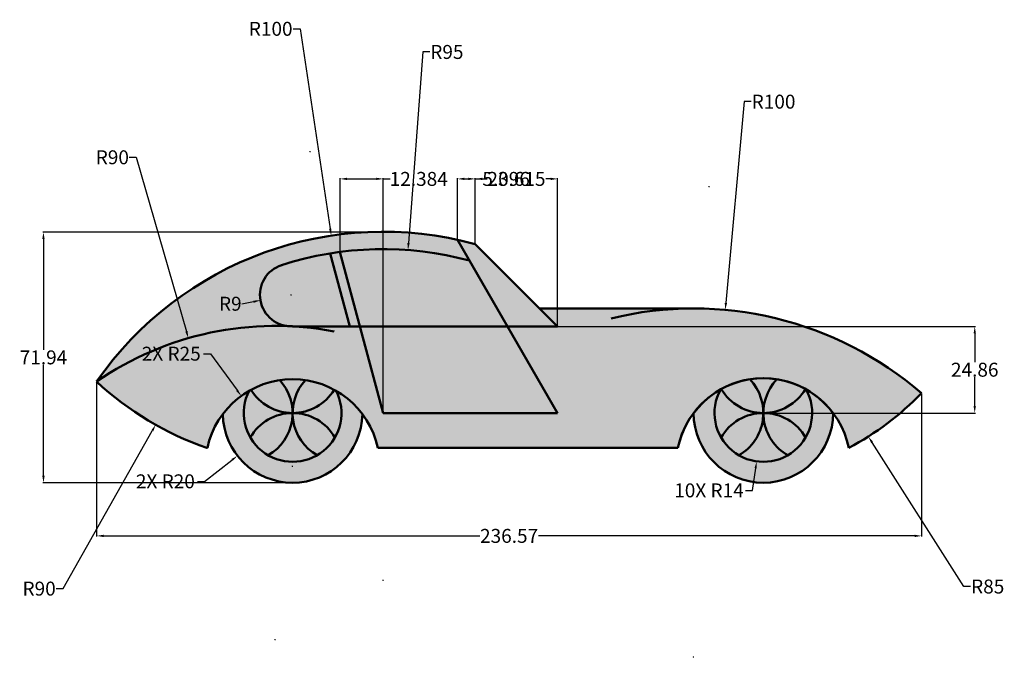
# Model space of a CAD drawing. Units: millimetres. Extents: x -64 to 541, y -54 to 145.
# Tile 2 of 2: x 259 to 541, y -43 to 140. Entities that reach past the tile are written whole.
import ezdxf

# ---------------------------------------------------------------- set-up
doc = ezdxf.new("R2010")
doc.units = ezdxf.units.MM
doc.header["$MEASUREMENT"] = 0
for name, color, linetype, lineweight in [('M-DIMS', 2, 'Continuous', 25), ('M-HATC', 9, 'Continuous', 18), ('M-OUTL', 7, 'Continuous', 50)]:
    doc.layers.add(name, color=color, linetype=linetype, lineweight=lineweight)
doc.styles.get("Standard").update_dxf_attribs({"font": 'arial.ttf'})
doc.dimstyles.get("Standard").update_dxf_attribs({"dimtxt": 4, "dimasz": 2, "dimexe": 0.18, "dimexo": 0.0625, "dimgap": 0.09, "dimtad": 0, "dimtih": 1, "dimtoh": 1, "dimdec": 0, "dimzin": 0, "dimdsep": 46, "dimtxsty": 'Standard', "dimcen": 0.09, "dimadec": 0, "dimazin": 0, "dimtfac": 1, "dimtdec": 0, "dimtofl": 0, "dimtmove": 0, "dimatfit": 3, "dimfxl": 1, "dimtolj": 1, "dimtzin": 0, "dimarcsym": 0})

# ---------------------------------------------------------------- blocks, each defined once
blk = doc.blocks.new('SPORTS-CAR-SIDE-PROFILE')
for p, q in [((132.2, 20), (103.49, 69.73)), ((132.2, 44.86), (108.59, 68.48)), ((72.59, 44.86), (66.98, 65.8)), ((82.17, 20), (69.79, 66.22)), ((171.2, 50), (127.07, 50)), ((56.2, 44.86), (132.2, 44.86)), ((82.17, 20), (132.2, 20)), ((31.62, 10), (31.77, 10)), ((80.64, 10), (166.71, 10))]:
    blk.add_line(p, q)
for centre, radius, start, end in [((82.17, -27.97), 100, 74.6835, 145.2591), ((82.17, -27.97), 95, 74.8819, 107.8414), ((55.83, 53.89), 9, 107.8414, 272.4141), ((171.2, -50), 100, 49.1795, 103.6939), ((51.2, -45), 90, 79.1521, 124.6758), ((61.2, 95), 90, 227.1529, 250.8119), ((56.2, 4.72), 25, 12.189, 167.811), ((42.2, 20), 14, 300, 42.4573), ((70.2, 20), 14, 137.5427, 240), ((191.2, 5), 25, 36.8699, 168.463), ((191.2, 5), 25, 11.537, 168.463), ((177.2, 20), 14, 300, 43.8229), ((205.2, 20), 14, 136.1771, 240), ((56.2, 20), 14, 152.7963, 27.2037), ((56.2, 34), 14, 211.4905, 328.5095), ((191.2, 20), 14, 150.9407, 29.0593), ((191.2, 34), 14, 210.4901, 329.5099), ((175.7, 85), 85, 298.0725, 315.739), ((56.2, 6), 14, 30, 150), ((191.2, 20), 20, 180, 0), ((191.2, 6), 14, 30, 150), ((56.2, 20), 20, 180.7904, 359.2096)]:
    blk.add_arc(centre, radius, start, end)
blk = doc.blocks.new('*D32')
at = {"layer": 'Defpoints', "color": 0, "transparency": 16777216}
for p in [(280.72, 35.85), (517.29, 32.51), (517.29, -8.41)]:
    blk.add_point(p, dxfattribs=at)
at = {"layer": 'M-DIMS', "color": 0, "lineweight": -2, "transparency": 16777216}
for p, q in [((280.72, 35.79), (280.72, -8.59)), ((517.29, 32.45), (517.29, -8.59)), ((282.72, -8.41), (390.58, -8.41)), ((515.29, -8.41), (407.43, -8.41))]:
    blk.add_line(p, q, dxfattribs=at)
at = {"layer": 'M-DIMS', "color": 0, "transparency": 16777216}
for points in [[(282.72, -8.08), (282.72, -8.75), (280.72, -8.41)], [(515.29, -8.08), (515.29, -8.75), (517.29, -8.41)]]:
    blk.add_solid(points, dxfattribs=at)
at = {"layer": 'M-DIMS', "color": 0, "transparency": 16777216, "insert": (399, -8.41), "char_height": 4, "attachment_point": 5}
blk.add_mtext('\\A1;236.57', dxfattribs=at)
blk = doc.blocks.new('*D33')
at = {"layer": 'Defpoints', "color": 0, "transparency": 16777216}
for p in [(265.47, 78.77), (358.48, 78.77), (336.92, 6.84)]:
    blk.add_point(p, dxfattribs=at)
at = {"layer": 'M-DIMS', "color": 0, "lineweight": -2, "transparency": 16777216}
for p, q in [((358.42, 78.77), (265.29, 78.77)), ((265.47, 76.77), (265.47, 44.94)), ((265.47, 8.84), (265.47, 40.67)), ((336.86, 6.84), (265.29, 6.84))]:
    blk.add_line(p, q, dxfattribs=at)
at = {"layer": 'M-DIMS', "color": 0, "transparency": 16777216}
for points in [[(265.13, 76.77), (265.8, 76.77), (265.47, 78.77)], [(265.13, 8.84), (265.8, 8.84), (265.47, 6.84)]]:
    blk.add_solid(points, dxfattribs=at)
at = {"layer": 'M-DIMS', "color": 0, "transparency": 16777216, "insert": (265.47, 42.81), "char_height": 4, "attachment_point": 5}
blk.add_mtext('\\A1;71.94', dxfattribs=at)
blk = doc.blocks.new('*D34')
at = {"layer": 'Defpoints', "color": 0, "transparency": 16777216}
for p in [(362.89, 94.02), (350.51, 73.05), (362.89, 26.84)]:
    blk.add_point(p, dxfattribs=at)
at = {"layer": 'M-DIMS', "color": 0, "lineweight": -2, "transparency": 16777216}
for p, q in [((350.51, 73.12), (350.51, 94.2)), ((352.51, 94.02), (360.89, 94.02)), ((362.89, 26.9), (362.89, 94.2)), ((362.89, 94.02), (364.89, 94.02))]:
    blk.add_line(p, q, dxfattribs=at)
at = {"layer": 'M-DIMS', "color": 0, "transparency": 16777216}
for points in [[(352.51, 94.36), (352.51, 93.69), (350.51, 94.02)], [(360.89, 94.36), (360.89, 93.69), (362.89, 94.02)]]:
    blk.add_solid(points, dxfattribs=at)
at = {"layer": 'M-DIMS', "color": 0, "transparency": 16777216, "insert": (373.09, 94.02), "char_height": 4, "attachment_point": 5}
blk.add_mtext('\\A1;12.384', dxfattribs=at)
blk = doc.blocks.new('*D35')
at = {"layer": 'Defpoints', "color": 0, "transparency": 16777216}
for p in [(389.31, 94.02), (384.21, 76.57), (389.31, 75.31)]:
    blk.add_point(p, dxfattribs=at)
at = {"layer": 'M-DIMS', "color": 0, "lineweight": -2, "transparency": 16777216}
for p, q in [((384.21, 76.63), (384.21, 94.2)), ((386.21, 94.02), (387.31, 94.02)), ((389.31, 75.38), (389.31, 94.2)), ((389.31, 94.02), (391.31, 94.02))]:
    blk.add_line(p, q, dxfattribs=at)
at = {"layer": 'M-DIMS', "color": 0, "transparency": 16777216}
for points in [[(386.21, 94.36), (386.21, 93.69), (384.21, 94.02)], [(387.31, 94.36), (387.31, 93.69), (389.31, 94.02)]]:
    blk.add_solid(points, dxfattribs=at)
at = {"layer": 'M-DIMS', "color": 0, "transparency": 16777216, "insert": (398.14, 94.02), "char_height": 4, "attachment_point": 5}
blk.add_mtext('\\A1;5.096', dxfattribs=at)
blk = doc.blocks.new('*D36')
at = {"layer": 'Defpoints', "color": 0, "transparency": 16777216}
for p in [(412.92, 94.02), (389.31, 75.31), (412.92, 51.7)]:
    blk.add_point(p, dxfattribs=at)
at = {"layer": 'M-DIMS', "color": 0, "lineweight": -2, "transparency": 16777216}
for p, q in [((389.31, 75.38), (389.31, 94.2)), ((391.31, 94.02), (392.67, 94.02)), ((410.92, 94.02), (409.55, 94.02)), ((412.92, 51.76), (412.92, 94.2))]:
    blk.add_line(p, q, dxfattribs=at)
at = {"layer": 'M-DIMS', "color": 0, "transparency": 16777216}
for points in [[(391.31, 94.36), (391.31, 93.69), (389.31, 94.02)], [(410.92, 94.36), (410.92, 93.69), (412.92, 94.02)]]:
    blk.add_solid(points, dxfattribs=at)
at = {"layer": 'M-DIMS', "color": 0, "transparency": 16777216, "insert": (401.11, 94.02), "char_height": 4, "attachment_point": 5}
blk.add_mtext('\\A1;23.615', dxfattribs=at)
blk = doc.blocks.new('*D37')
at = {"layer": 'Defpoints', "color": 0, "transparency": 16777216}
for p in [(412.92, 51.7), (532.54, 51.7), (471.92, 26.84)]:
    blk.add_point(p, dxfattribs=at)
at = {"layer": 'M-DIMS', "color": 0, "lineweight": -2, "transparency": 16777216}
for p, q in [((412.98, 51.7), (532.72, 51.7)), ((532.54, 49.7), (532.54, 41.4)), ((532.54, 28.84), (532.54, 37.14)), ((471.98, 26.84), (532.72, 26.84))]:
    blk.add_line(p, q, dxfattribs=at)
at = {"layer": 'M-DIMS', "color": 0, "transparency": 16777216}
for points in [[(532.21, 49.7), (532.87, 49.7), (532.54, 51.7)], [(532.21, 28.84), (532.87, 28.84), (532.54, 26.84)]]:
    blk.add_solid(points, dxfattribs=at)
at = {"layer": 'M-DIMS', "color": 0, "transparency": 16777216, "insert": (532.54, 39.27), "char_height": 4, "attachment_point": 5}
blk.add_mtext('\\A1;24.86', dxfattribs=at)
blk = doc.blocks.new('*D38')
at = {"layer": 'Defpoints', "color": 0, "transparency": 16777216}
for p in [(322.18, 31.75), (336.92, 11.56)]:
    blk.add_point(p, dxfattribs=at)
at = {"layer": 'M-DIMS', "color": 0, "lineweight": -2, "transparency": 16777216}
for p, q in [((311.34, 43.87), (313.34, 43.87)), ((313.34, 43.87), (321, 33.37)), ((336.83, 11.56), (337.01, 11.56)), ((336.92, 11.47), (336.92, 11.65))]:
    blk.add_line(p, q, dxfattribs=at)
at = {"layer": 'M-DIMS', "color": 0, "transparency": 16777216}
blk.add_solid([(321.27, 33.56), (320.73, 33.17), (322.18, 31.75)], dxfattribs=at)
at = {"layer": 'M-DIMS', "color": 0, "transparency": 16777216, "insert": (302.12, 43.87), "char_height": 4, "attachment_point": 5}
blk.add_mtext('\\A1;2X R25', dxfattribs=at)
blk = doc.blocks.new('*D39')
at = {"layer": 'Defpoints', "color": 0, "transparency": 16777216}
for p in [(336.92, 26.84), (321.11, 14.59)]:
    blk.add_point(p, dxfattribs=at)
at = {"layer": 'M-DIMS', "color": 0, "lineweight": -2, "transparency": 16777216}
for p, q in [((336.83, 26.84), (337.01, 26.84)), ((336.92, 26.75), (336.92, 26.93)), ((311.63, 7.24), (319.53, 13.36)), ((309.63, 7.24), (311.63, 7.24))]:
    blk.add_line(p, q, dxfattribs=at)
at = {"layer": 'M-DIMS', "color": 0, "transparency": 16777216}
blk.add_solid([(319.33, 13.62), (319.73, 13.1), (321.11, 14.59)], dxfattribs=at)
at = {"layer": 'M-DIMS', "color": 0, "transparency": 16777216, "insert": (300.43, 7.24), "char_height": 4, "attachment_point": 5}
blk.add_mtext('\\A1;2X R20', dxfattribs=at)
blk = doc.blocks.new('*D40')
at = {"layer": 'Defpoints', "color": 0, "transparency": 16777216}
for p in [(471.92, 26.84), (470, 12.97)]:
    blk.add_point(p, dxfattribs=at)
at = {"layer": 'M-DIMS', "color": 0, "lineweight": -2, "transparency": 16777216}
for p, q in [((471.83, 26.84), (472.01, 26.84)), ((471.92, 26.75), (471.92, 26.93)), ((468.84, 4.65), (469.72, 10.99)), ((466.84, 4.65), (468.84, 4.65))]:
    blk.add_line(p, q, dxfattribs=at)
at = {"layer": 'M-DIMS', "color": 0, "transparency": 16777216}
blk.add_solid([(469.39, 11.04), (470.05, 10.94), (470, 12.97)], dxfattribs=at)
at = {"layer": 'M-DIMS', "color": 0, "transparency": 16777216, "insert": (456.32, 4.65), "char_height": 4, "attachment_point": 5}
blk.add_mtext('\\A1;10X R14', dxfattribs=at)
blk = doc.blocks.new('*D41')
at = {"layer": 'Defpoints', "color": 0, "transparency": 16777216}
for p in [(336.54, 60.73), (327.68, 59.15)]:
    blk.add_point(p, dxfattribs=at)
at = {"layer": 'M-DIMS', "color": 0, "lineweight": -2, "transparency": 16777216}
for p, q in [((336.45, 60.73), (336.63, 60.73)), ((336.54, 60.64), (336.54, 60.82)), ((322.37, 58.2), (325.71, 58.8))]:
    blk.add_line(p, q, dxfattribs=at)
at = {"layer": 'M-DIMS', "color": 0, "transparency": 16777216}
blk.add_solid([(325.65, 59.12), (325.77, 58.47), (327.68, 59.15)], dxfattribs=at)
at = {"layer": 'M-DIMS', "color": 0, "transparency": 16777216, "insert": (319.05, 58.2), "char_height": 4, "attachment_point": 5}
blk.add_mtext('\\A1;R9', dxfattribs=at)
blk = doc.blocks.new('*D42')
at = {"layer": 'Defpoints', "color": 0, "transparency": 16777216}
for p in [(347.99, 77.75), (362.89, -21.13)]:
    blk.add_point(p, dxfattribs=at)
at = {"layer": 'M-DIMS', "color": 0, "lineweight": -2, "transparency": 16777216}
for p, q in [((337.04, 137.08), (339.04, 137.08)), ((339.04, 137.08), (347.69, 79.73)), ((362.8, -21.13), (362.98, -21.13)), ((362.89, -21.22), (362.89, -21.04))]:
    blk.add_line(p, q, dxfattribs=at)
at = {"layer": 'M-DIMS', "color": 0, "transparency": 16777216}
blk.add_solid([(348.02, 79.78), (347.36, 79.68), (347.99, 77.75)], dxfattribs=at)
at = {"layer": 'M-DIMS', "color": 0, "transparency": 16777216, "insert": (330.63, 137.08), "char_height": 4, "attachment_point": 5}
blk.add_mtext('\\A1;R100', dxfattribs=at)
blk = doc.blocks.new('*D43')
at = {"layer": 'Defpoints', "color": 0, "transparency": 16777216}
for p in [(370.01, 73.6), (362.89, -21.13)]:
    blk.add_point(p, dxfattribs=at)
at = {"layer": 'M-DIMS', "color": 0, "lineweight": -2, "transparency": 16777216}
for p, q in [((374.28, 130.44), (370.16, 75.59)), ((376.28, 130.44), (374.28, 130.44)), ((362.8, -21.13), (362.98, -21.13)), ((362.89, -21.22), (362.89, -21.04))]:
    blk.add_line(p, q, dxfattribs=at)
at = {"layer": 'M-DIMS', "color": 0, "transparency": 16777216}
blk.add_solid([(369.82, 75.62), (370.49, 75.57), (370.01, 73.6)], dxfattribs=at)
at = {"layer": 'M-DIMS', "color": 0, "transparency": 16777216, "insert": (381.16, 130.44), "char_height": 4, "attachment_point": 5}
blk.add_mtext('\\A1;R95', dxfattribs=at)
blk = doc.blocks.new('*D44')
at = {"layer": 'Defpoints', "color": 0, "transparency": 16777216}
for p in [(307.02, 48.32), (331.92, -38.16)]:
    blk.add_point(p, dxfattribs=at)
at = {"layer": 'M-DIMS', "color": 0, "lineweight": -2, "transparency": 16777216}
for p, q in [((290.08, 100.22), (292.08, 100.22)), ((292.08, 100.22), (306.47, 50.25)), ((331.83, -38.16), (332.01, -38.16)), ((331.92, -38.25), (331.92, -38.07))]:
    blk.add_line(p, q, dxfattribs=at)
at = {"layer": 'M-DIMS', "color": 0, "transparency": 16777216}
blk.add_solid([(306.79, 50.34), (306.15, 50.15), (307.02, 48.32)], dxfattribs=at)
at = {"layer": 'M-DIMS', "color": 0, "transparency": 16777216, "insert": (285.22, 100.22), "char_height": 4, "attachment_point": 5}
blk.add_mtext('\\A1;R90', dxfattribs=at)
blk = doc.blocks.new('*D45')
at = {"layer": 'Defpoints', "color": 0, "transparency": 16777216}
for p in [(341.92, 101.84), (297.65, 23.48)]:
    blk.add_point(p, dxfattribs=at)
at = {"layer": 'M-DIMS', "color": 0, "lineweight": -2, "transparency": 16777216}
for p, q in [((341.83, 101.84), (342.01, 101.84)), ((341.92, 101.75), (341.92, 101.93)), ((271.09, -23.54), (296.67, 21.74)), ((269.09, -23.54), (271.09, -23.54))]:
    blk.add_line(p, q, dxfattribs=at)
at = {"layer": 'M-DIMS', "color": 0, "transparency": 16777216}
blk.add_solid([(296.38, 21.9), (296.96, 21.57), (297.65, 23.48)], dxfattribs=at)
at = {"layer": 'M-DIMS', "color": 0, "transparency": 16777216, "insert": (264.22, -23.54), "char_height": 4, "attachment_point": 5}
blk.add_mtext('\\A1;R90', dxfattribs=at)
blk = doc.blocks.new('*D46')
at = {"layer": 'Defpoints', "color": 0, "transparency": 16777216}
for p in [(460.99, 56.43), (451.92, -43.16)]:
    blk.add_point(p, dxfattribs=at)
at = {"layer": 'M-DIMS', "color": 0, "lineweight": -2, "transparency": 16777216}
for p, q in [((466.44, 116.18), (461.17, 58.42)), ((468.44, 116.18), (466.44, 116.18)), ((451.83, -43.16), (452.01, -43.16)), ((451.92, -43.25), (451.92, -43.07))]:
    blk.add_line(p, q, dxfattribs=at)
at = {"layer": 'M-DIMS', "color": 0, "transparency": 16777216}
blk.add_solid([(460.84, 58.45), (461.51, 58.39), (460.99, 56.43)], dxfattribs=at)
at = {"layer": 'M-DIMS', "color": 0, "transparency": 16777216, "insert": (474.85, 116.18), "char_height": 4, "attachment_point": 5}
blk.add_mtext('\\A1;R100', dxfattribs=at)
blk = doc.blocks.new('*D47')
at = {"layer": 'Defpoints', "color": 0, "transparency": 16777216}
for p in [(456.42, 91.84), (502.01, 20.1)]:
    blk.add_point(p, dxfattribs=at)
at = {"layer": 'M-DIMS', "color": 0, "lineweight": -2, "transparency": 16777216}
for p, q in [((456.33, 91.84), (456.51, 91.84)), ((456.42, 91.75), (456.42, 91.93)), ((529.37, -22.94), (503.09, 18.42)), ((531.37, -22.94), (529.37, -22.94))]:
    blk.add_line(p, q, dxfattribs=at)
at = {"layer": 'M-DIMS', "color": 0, "transparency": 16777216}
blk.add_solid([(503.37, 18.59), (502.81, 18.24), (502.01, 20.1)], dxfattribs=at)
at = {"layer": 'M-DIMS', "color": 0, "transparency": 16777216, "insert": (536.26, -22.94), "char_height": 4, "attachment_point": 5}
blk.add_mtext('\\A1;R85', dxfattribs=at)

msp = doc.modelspace()

# ---------------------------------------------------------------- hatches: boundary and pattern name
at = {"layer": 'M-HATC'}
h = msp.add_hatch(color=256, dxfattribs=at)
h.dxf.hatch_style = 1
h.paths.add_polyline_path([(333.7838, 69.2968, -0.14481235), (387.667, 70.5776), (384.2092, 76.5666, 0.30367332), (280.7164, 35.8521, -0.16443349), (336.1211, 51.7394, -0.83526516)])
h.paths.add_polyline_path([(389.3052, 75.3137, 0.01312154), (384.2092, 76.5666), (387.667, 70.5776), (398.5668, 51.6985), (412.9203, 51.6985)])
h = msp.add_hatch(color=256, dxfattribs=at)
h.dxf.hatch_style = 1
h.paths.add_polyline_path([(353.3101, 51.6985), (347.6981, 72.6429, 0.03771409), (333.7838, 69.2968, 0.83526516), (336.1211, 51.7394, -0.00222284), (336.9203, 51.6985)])
h.paths.add_polyline_path([(398.5668, 51.6985), (387.667, 70.5776, 0.09896843), (350.5062, 73.0549), (356.2287, 51.6985)])
h = msp.add_hatch(color=256, dxfattribs=at)
h.dxf.hatch_style = 1
h.paths.add_polyline_path([(350.5062, 73.0549, 0.00746935), (347.6981, 72.6429), (353.3101, 51.6985), (356.2287, 51.6985)])
h = msp.add_hatch(color=256, dxfattribs=at)
h.dxf.hatch_style = 1
h.paths.add_polyline_path([(451.9203, 56.8375), (407.7813, 56.8375), (412.9203, 51.6985), (398.5668, 51.6985), (412.9203, 26.8375), (362.8901, 26.8375), (356.2287, 51.6985), (336.9203, 51.6985, 0.16671727), (280.7164, 35.8521, 0.10359983), (312.3399, 16.8375), (312.4839, 16.8375, -0.80705656), (361.3567, 16.8375), (447.4254, 16.8375, -0.81649658), (496.4152, 16.8375, 0.07723768), (517.2895, 32.5136, 0.1800208)])
h.paths.add_polyline_path([(398.5668, 51.6985), (356.2287, 51.6985), (362.8901, 26.8375), (412.9203, 26.8375)], flags=17)
h = msp.add_hatch(color=256, dxfattribs=at)
h.dxf.hatch_style = 1
h.paths.add_polyline_path([(451.9203, 56.8375), (407.7813, 56.8375), (412.9203, 51.6985), (398.5668, 51.6985), (412.9203, 26.8375), (362.8901, 26.8375), (356.2287, 51.6985), (336.9203, 51.6985, 0.16671727), (280.7164, 35.8521, 0.10359983), (312.3399, 16.8375), (312.4839, 16.8375, -0.80705656), (361.3567, 16.8375), (447.4254, 16.8375, -0.81649658), (496.4152, 16.8375, 0.07723768), (517.2895, 32.5136, 0.1800208)])
h = msp.add_hatch(color=256, dxfattribs=at)
h.dxf.hatch_style = 1
h.paths.add_polyline_path([(356.2287, 51.6985), (362.8901, 26.8375), (412.9203, 26.8375), (398.5668, 51.6985)])
h = msp.add_hatch(color=256, dxfattribs=at)
h.dxf.hatch_style = 1
h.paths.add_polyline_path([(356.2287, 51.6985), (362.8901, 26.8375), (412.9203, 26.8375), (398.5668, 51.6985)])
h = msp.add_hatch(color=256, dxfattribs=at)
h.dxf.hatch_style = 1
h.paths.add_polyline_path([(356.9184, 26.5616, 0.10180257), (349.3717, 33.2377, -1.63838242), (324.4689, 33.2377, 0.10180257), (316.9222, 26.5616, 0.98629895)])
h.paths.add_polyline_path([(459.6827, 33.6375, 0.10431902), (451.9203, 26.8375, 1), (491.9203, 26.8375, 0.10431902), (484.158, 33.6375, -1.69967317)])
h.paths.add_polyline_path([(343.9203, 14.7132, -0.26794919), (336.9203, 26.8375, -0.26794919), (329.9203, 14.7132, 0.26794919)], flags=17)
h.paths.add_polyline_path([(336.9203, 26.8375, -0.26099062), (324.9821, 33.5245, 0.00587967), (324.4689, 33.2377, 0.25491407), (324.796, 19.8375, -0.26794919)])
h.paths.add_polyline_path([(340.5914, 36.2881, 0.07382143), (333.2492, 36.2881, -0.18740354), (336.9203, 26.8375, -0.18740354)])
h.paths.add_polyline_path([(349.3717, 33.2377, 0.00587967), (348.8585, 33.5245, -0.26099062), (336.9203, 26.8375, -0.26794919), (349.0447, 19.8375, 0.25491407)])
h.paths.add_polyline_path([(471.9203, 26.8375, -0.26794919), (464.9203, 14.7132, 0.26794919), (478.9203, 14.7132, -0.26794919)], flags=17)
h.paths.add_polyline_path([(471.9203, 26.8375, -0.2656586), (459.8563, 33.7341, 0.00198652), (459.6827, 33.6375, 0.26355464), (459.796, 19.8375, -0.26794919)])
h.paths.add_polyline_path([(475.8196, 36.5316, 0.07846483), (468.0211, 36.5316, -0.19357861), (471.9203, 26.8375, -0.19357861)])
h.paths.add_polyline_path([(484.158, 33.6375, 0.00198652), (483.9844, 33.7341, -0.2656586), (471.9203, 26.8375, -0.26794919), (484.0447, 19.8375, 0.26355464)])
h = msp.add_hatch(color=256, dxfattribs=at)
h.dxf.hatch_style = 1
h.paths.add_polyline_path([(336.9203, 26.8375, 0.18740354), (333.2492, 36.2881, 0.08784044), (324.9821, 33.5245, 0.26099062)])
h.paths.add_polyline_path([(336.9203, 26.8375, 0.26794919), (324.796, 19.8375, 0.1316525), (329.9203, 14.7132, 0.26794919)])
h.paths.add_polyline_path([(349.0447, 19.8375, 0.26794919), (336.9203, 26.8375, 0.26794919), (343.9203, 14.7132, 0.1316525)])
h.paths.add_polyline_path([(348.8585, 33.5245, 0.08784044), (340.5914, 36.2881, 0.18740354), (336.9203, 26.8375, 0.26099062)])
h.paths.add_polyline_path([(471.9203, 26.8375, 0.26794919), (459.796, 19.8375, 0.1316525), (464.9203, 14.7132, 0.26794919)])
h.paths.add_polyline_path([(468.0211, 36.5316, 0.08696025), (459.8563, 33.7341, 0.2656586), (471.9203, 26.8375, 0.19357861)])
h.paths.add_polyline_path([(483.9844, 33.7341, 0.08696025), (475.8196, 36.5316, 0.19357861), (471.9203, 26.8375, 0.2656586)])
h.paths.add_polyline_path([(478.9203, 14.7132, 0.1316525), (484.0447, 19.8375, 0.26794919), (471.9203, 26.8375, 0.26794919)])
h = msp.add_hatch(color=256, dxfattribs=at)
h.dxf.hatch_style = 1
h.paths.add_polyline_path([(348.8585, 33.5245, 0.08784044), (340.5914, 36.2881, 0.18740354), (336.9203, 26.8375, 0.26099062)])
h.paths.add_polyline_path([(349.0447, 19.8375, 0.26794919), (336.9203, 26.8375, 0.26794919), (343.9203, 14.7132, 0.1316525)])
h.paths.add_polyline_path([(336.9203, 26.8375, 0.26794919), (324.796, 19.8375, 0.1316525), (329.9203, 14.7132, 0.26794919)])
h.paths.add_polyline_path([(333.2492, 36.2881, 0.08784044), (324.9821, 33.5245, 0.26099062), (336.9203, 26.8375, 0.18740354)])
h.paths.add_polyline_path([(471.9203, 26.8375, 0.26794919), (478.9203, 14.7132, 0.1316525), (484.0447, 19.8375, 0.26794919)])
h.paths.add_polyline_path([(483.9844, 33.7341, 0.08696025), (475.8196, 36.5316, 0.19357861), (471.9203, 26.8375, 0.2656586)])
h.paths.add_polyline_path([(468.0211, 36.5316, 0.08696025), (459.8563, 33.7341, 0.2656586), (471.9203, 26.8375, 0.19357861)])
h.paths.add_polyline_path([(471.9203, 26.8375, 0.26794919), (459.796, 19.8375, 0.1316525), (464.9203, 14.7132, 0.26794919)])

# ---------------------------------------------------------------- block references
at = {"layer": 'M-OUTL'}
msp.add_blockref('SPORTS-CAR-SIDE-PROFILE', (280.7159, 6.838), dxfattribs=at)

# ---------------------------------------------------------------- dimensions: what is measured, and where the dimension line sits
at = {"layer": 'M-DIMS'}
for center, mpoint, picture, middle in [((362.8901, -21.1345), (347.9852, 77.7485), '*D42', (330.6261, 137.0783)), ((362.8901, -21.1345), (370.0074, 73.5985), '*D43', (381.1618, 130.4383)), ((451.9203, -43.1625), (460.9932, 56.4251), '*D46', (474.8529, 116.1776)), ((341.9203, 101.8375), (297.6491, 23.479), '*D45', (264.2243, -23.5362)), ((331.9203, -38.1625), (307.0216, 48.3248), '*D44', (285.2203, 100.2172)), ((456.4152, 91.8375), (502.0145, 20.104), '*D47', (536.2581, -22.9361)), ((336.5412, 60.7296), (327.6815, 59.1471), '*D41', (322.3656, 58.1976))]:
    dim = msp.add_radius_dim(center=center, mpoint=mpoint, dimstyle='Standard', override={"dimdec": 0, "dimlfac": 1, "dimrnd": 0, "dimzin": 0, "dimdsep": 46, "dimlunit": 2}, dxfattribs=at)
    dim.commit()
    dim.dimension.update_dxf_attribs({"geometry": picture, "text_midpoint": middle, "dimtype": 164})
for base, p1, p2, override, picture, middle in [((362.8901, 94.0243), (350.5062, 73.0549), (362.8901, 26.8375), {"dimdec": 3, "dimlfac": 1, "dimrnd": 0, "dimzin": 0, "dimdsep": 46, "dimlunit": 2}, '*D34', (373.0866, 94.0243)), ((389.3052, 94.0243), (384.2092, 76.5666), (389.3052, 75.3137), {"dimdec": 3, "dimlfac": 1, "dimrnd": 0, "dimzin": 0, "dimdsep": 46, "dimlunit": 2}, '*D35', (398.1428, 94.0243)), ((412.9203, 94.0243), (389.3052, 75.3137), (412.9203, 51.6985), {"dimdec": 3, "dimlfac": 1, "dimrnd": 0, "dimzin": 0, "dimdsep": 46, "dimlunit": 2}, '*D36', (401.1128, 94.0243)), ((517.2895, -8.4125), (280.7164, 35.8521), (517.2895, 32.5136), {"dimdec": 2, "dimlfac": 1, "dimrnd": 0, "dimzin": 0, "dimdsep": 46, "dimlunit": 2}, '*D32', (399.0029, -8.4125))]:
    dim = msp.add_linear_dim(base=base, p1=p1, p2=p2, dimstyle='Standard', override=override, dxfattribs=at)
    dim.commit()
    dim.dimension.update_dxf_attribs({"geometry": picture, "text_midpoint": middle})
for base, p1, p2, picture, middle in [((265.4664, 78.7743), (336.9203, 6.8375), (358.4811, 78.7743), '*D33', (265.4664, 42.8059)), ((532.5395, 51.6985), (471.9203, 26.8375), (412.9203, 51.6985), '*D37', (532.5395, 39.268))]:
    dim = msp.add_linear_dim(base=base, p1=p1, p2=p2, angle=90, dimstyle='Standard', override={"dimdec": 2, "dimlfac": 1, "dimrnd": 0, "dimzin": 0, "dimdsep": 46, "dimlunit": 2}, dxfattribs=at)
    dim.commit()
    dim.dimension.update_dxf_attribs({"geometry": picture, "text_midpoint": middle})
for center, mpoint, text, picture, middle in [((336.9203, 11.5591), (322.181, 31.752), '2X <>', '*D38', (302.1219, 43.8677)), ((336.9203, 26.8375), (321.1117, 14.5865), '2X <>', '*D39', (300.4328, 7.2359)), ((471.9203, 26.8375), (469.9959, 12.9704), '10X <>', '*D40', (456.3174, 4.6502))]:
    dim = msp.add_radius_dim(center=center, mpoint=mpoint, text=text, dimstyle='Standard', override={"dimdec": 0, "dimlfac": 1, "dimrnd": 0, "dimzin": 0, "dimdsep": 46, "dimlunit": 2}, dxfattribs=at)
    dim.commit()
    dim.dimension.update_dxf_attribs({"geometry": picture, "text_midpoint": middle, "dimtype": 164})

doc.saveas('drawing.dxf')
